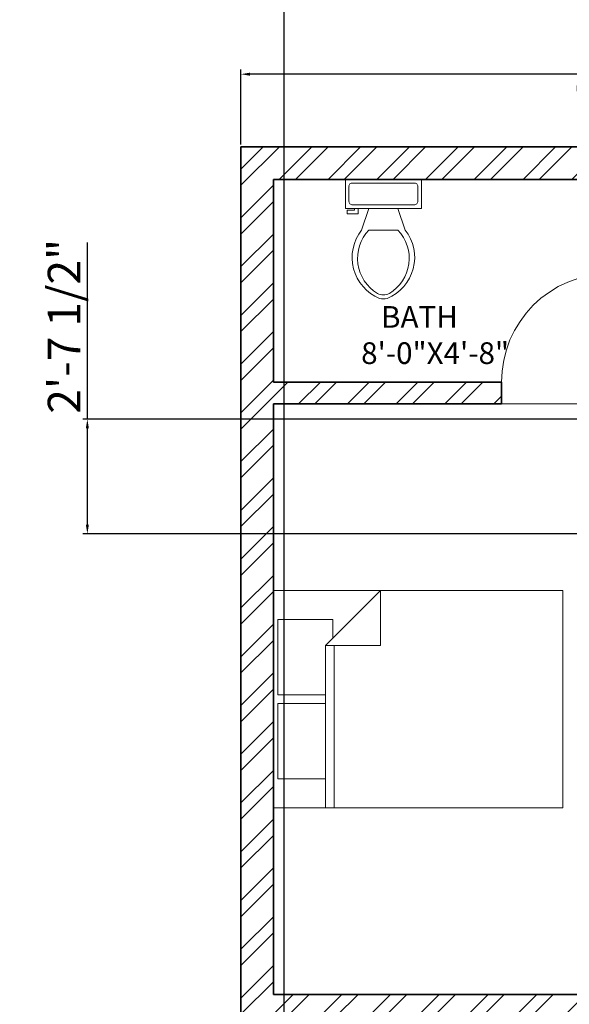
# Model space of a CAD drawing. Units: inches. Extents: x 744 to 1448, y 5126 to 6077.
# Tile 5 of 10: x 744 to 895, y 5585 to 5857. Entities that reach past the tile are written whole.
import ezdxf

# ---------------------------------------------------------------- set-up
doc = ezdxf.new("R2010")
doc.units = ezdxf.units.IN
for name, color, linetype, lineweight in [('A-ANNO-DIMS', 2, 'Continuous', 18), ('A-AREA-IDEN', 7, 'Continuous', 18), ('A-DOOR', 4, 'Continuous', 18), ('A-FLOR-FIXT', 9, 'Continuous', 18), ('A-FURN', 8, 'Continuous', 18), ('A-WALL', 7, 'Continuous', 35), ('A-WALL-PATT', 252, 'Continuous', 13)]:
    doc.layers.add(name, color=color, linetype=linetype, lineweight=lineweight)
doc.styles.get("Standard").update_dxf_attribs({"font": 'arial.ttf'})
doc.dimstyles.new('ISO-25', dxfattribs={"dimtxt": 9, "dimasz": 2.5, "dimexe": 1.25, "dimexo": 0.625, "dimtad": 1, "dimlunit": 3, "dimtxsty": 'Standard', "dimcen": 2.5, "dimadec": 0, "dimazin": 0, "dimtfac": 1, "dimtmove": 0, "dimatfit": 3, "dimfxl": 1, "dimarcsym": 0})

# ---------------------------------------------------------------- blocks, each defined once
blk = doc.blocks.new('*U4')
for p, q in [((0, 0), (0, 6)), ((40, 0), (40, 6))]:
    blk.add_line(p, q)
blk.add_lwpolyline([(0, 0), (0, -40), (1.75, -40), (1.75, 0)], close=True)
blk.add_arc((0, 0), 40, 270, 0)
blk = doc.blocks.new('*U8')
for p, q in [((9.5, -6), (9.5, -2)), ((-8, -8.5), (-8, -8)), ((-7, -8), (-7, -9.5)), ((-4, -8), (-6, -14)), ((4, -8), (6, -14)), ((-10, -8.5), (-8, -8.5)), ((-10, -9.5), (-10, -8.5)), ((-7, -9.5), (-10, -9.5)), ((4, -14), (-4, -14))]:
    blk.add_line(p, q)
blk.add_lwpolyline([(10.5, -8), (10.5, 0), (-10.5, 0), (-10.5, -8)], close=True)
for points in [[(-9.5, -2), (-9.5, -6)], [(8.5, -1), (-8.5, -1)], [(-8.5, -7), (8.5, -7)]]:
    blk.add_lwpolyline(points)
for centre, radius, start, end in [((-8.62, -1.88), 0.884, 81.8699, 188.1301), ((8.62, -1.88), 0.884, 351.8699, 98.1301), ((-8.62, -6.12), 0.884, 171.8699, 278.1301), ((8.62, -6.12), 0.884, 261.8699, 8.1301), ((3.52, -21.58), 12.17, 141.4691, 247.9714), ((4.2, -21.82), 11.33, 136.3677, 238.9468), ((-3.52, -21.58), 12.17, 292.0284, 38.5307), ((-4.2, -21.82), 11.33, 301.053, 43.6321), ((0, -27.88), 4, 245.7318, 294.2682), ((0, -29), 4, 254.8605, 285.1395)]:
    blk.add_arc(centre, radius, start, end)
blk = doc.blocks.new('Bed - Queen')
for p, q in [((0, -80.00003), (0, 0)), ((0, 0), (59.99999, 0)), ((59.99999, 0), (59.99999, -80.00003)), ((7.99999, -1.2), (28.79998, -1.2)), ((7.99999, -14.4), (7.99999, -1.2)), ((28.79998, -1.2), (28.79998, -14.4)), ((31.19999, -1.2), (51.99999, -1.2)), ((31.19999, -14.4), (31.19999, -1.2)), ((51.99999, -1.2), (51.99999, -16.4)), ((0, -14.4), (44.8, -14.4)), ((59.99999, -29.6), (44.8, -14.4)), ((44.8, -14.4), (44.8, -29.6)), ((44.8, -16.8), (0, -16.8)), ((51.99999, -16.4), (46.79936, -16.4)), ((44.8, -29.6), (59.99999, -29.6)), ((59.99999, -80.00003), (0, -80.00003))]:
    blk.add_line(p, q)
blk = doc.blocks.new('*D24')
at = {"layer": 'A-ANNO-DIMS', "color": 0, "lineweight": -2, "transparency": 16777216}
for p, q in [((804.68, 5822.44), (804.68, 5843.13)), ((1320.68, 5822.44), (1320.68, 5843.13)), ((1318.18, 5841.88), (807.18, 5841.88))]:
    blk.add_line(p, q, dxfattribs=at)
at = {"layer": 'A-ANNO-DIMS', "color": 0, "transparency": 16777216}
for points in [[(807.18, 5842.3), (807.18, 5841.46), (804.68, 5841.88)], [(1318.18, 5842.3), (1318.18, 5841.46), (1320.68, 5841.88)]]:
    blk.add_solid(points, dxfattribs=at)
at = {"layer": 'Defpoints', "color": 0, "transparency": 16777216}
for p in [(804.68, 5841.88), (804.68, 5821.82), (1320.68, 5821.82)]:
    blk.add_point(p, dxfattribs=at)
at = {"layer": 'A-ANNO-DIMS', "color": 0, "transparency": 16777216, "insert": (1062.68, 5847.1), "char_height": 9, "attachment_point": 5}
blk.add_mtext("43'", dxfattribs=at)
blk = doc.blocks.new('*D41')
at = {"layer": 'A-ANNO-DIMS', "color": 0, "lineweight": -2, "transparency": 16777216}
for p, q in [((908.53, 5795.32), (908.53, 5925.53)), ((911.06, 5795.32), (907.28, 5795.32)), ((908.53, 5776.82), (908.53, 5792.82)), ((911.06, 5774.32), (907.28, 5774.32))]:
    blk.add_line(p, q, dxfattribs=at)
at = {"layer": 'A-ANNO-DIMS', "color": 0, "transparency": 16777216}
for points in [[(908.12, 5792.82), (908.95, 5792.82), (908.53, 5795.32)], [(908.12, 5776.82), (908.95, 5776.82), (908.53, 5774.32)]]:
    blk.add_solid(points, dxfattribs=at)
at = {"layer": 'Defpoints', "color": 0, "transparency": 16777216}
for p in [(908.53, 5795.32), (911.68, 5795.32), (911.68, 5774.32)]:
    blk.add_point(p, dxfattribs=at)
at = {"layer": 'A-ANNO-DIMS', "color": 0, "transparency": 16777216, "insert": (903.25, 5861.67), "char_height": 9, "attachment_point": 5, "rotation": 90}
blk.add_mtext('WINDOW C 1\'-9" TYP.', dxfattribs=at)
blk = doc.blocks.new('*D59')
at = {"layer": 'A-ANNO-DIMS', "color": 0, "lineweight": -2, "transparency": 16777216}
for p, q in [((762.28, 5746.58), (762.28, 5795.38)), ((1128.24, 5746.58), (761.03, 5746.58)), ((762.28, 5717.4), (762.28, 5744.08)), ((1128.24, 5714.9), (761.03, 5714.9))]:
    blk.add_line(p, q, dxfattribs=at)
at = {"layer": 'A-ANNO-DIMS', "color": 0, "transparency": 16777216}
for points in [[(761.87, 5744.08), (762.7, 5744.08), (762.28, 5746.58)], [(761.87, 5717.4), (762.7, 5717.4), (762.28, 5714.9)]]:
    blk.add_solid(points, dxfattribs=at)
at = {"layer": 'Defpoints', "color": 0, "transparency": 16777216}
for p in [(762.28, 5746.58), (1128.86, 5746.58), (1128.86, 5714.9)]:
    blk.add_point(p, dxfattribs=at)
at = {"layer": 'A-ANNO-DIMS', "color": 0, "transparency": 16777216, "insert": (757.01, 5772.23), "char_height": 9, "attachment_point": 5, "rotation": 90}
blk.add_mtext('2\'-7 1/2"', dxfattribs=at)
blk = doc.blocks.new('*D62')
at = {"layer": 'A-ANNO-DIMS', "color": 0, "lineweight": -2, "transparency": 16777216}
for p, q in [((816.68, 5262.94), (816.68, 6059.61)), ((819.18, 6058.36), (974.68, 6058.36)), ((977.18, 5262.94), (977.18, 6059.61))]:
    blk.add_line(p, q, dxfattribs=at)
at = {"layer": 'A-ANNO-DIMS', "color": 0, "transparency": 16777216}
for points in [[(819.18, 6058.78), (819.18, 6057.95), (816.68, 6058.36)], [(974.68, 6058.78), (974.68, 6057.95), (977.18, 6058.36)]]:
    blk.add_solid(points, dxfattribs=at)
at = {"layer": 'Defpoints', "color": 0, "transparency": 16777216}
for p in [(977.18, 6058.36), (816.68, 5262.32), (977.18, 5262.32)]:
    blk.add_point(p, dxfattribs=at)
at = {"layer": 'A-ANNO-DIMS', "color": 0, "transparency": 16777216, "insert": (896.93, 6063.64), "char_height": 9, "attachment_point": 5}
blk.add_mtext('13\'-4 1/2"', dxfattribs=at)

msp = doc.modelspace()

# ---------------------------------------------------------------- hatches: boundary and pattern name
at = {"layer": 'A-WALL-PATT'}
h = msp.add_hatch(dxfattribs=at)
h.set_pattern_fill('ANSI32', color=256)
h.paths.add_polyline_path([(813.684, 5750.816), (876.684, 5750.816), (876.684, 5756.816), (813.684, 5756.816), (813.684, 5812.816), (909.684, 5812.816), (909.684, 5795.316), (915.684, 5795.316), (915.684, 5812.816), (1209.684, 5812.816), (1209.684, 5795.316), (1215.684, 5795.316), (1215.684, 5812.816), (1311.684, 5812.816), (1311.684, 5756.816), (1248.684, 5756.816), (1248.684, 5750.816), (1311.684, 5750.816), (1311.684, 5570.816), (1179.044, 5570.816), (1179.044, 5564.816), (1311.684, 5564.816), (1311.684, 5383.316), (1260.684, 5383.316), (1260.684, 5377.316), (1311.684, 5377.316), (1311.684, 5320.316), (1227.684, 5320.316), (1227.684, 5333.816), (1221.684, 5333.816), (1221.684, 5314.316), (1320.684, 5314.316), (1320.684, 5821.816), (804.684, 5821.816), (804.684, 5472.316), (926.184, 5472.316), (926.184, 5481.316), (813.684, 5481.316), (813.684, 5581.616), (946.284, 5581.616), (946.284, 5587.616), (813.684, 5587.616)])
h.paths.add_polyline_path([(1155.684, 5525.816), (1149.684, 5525.816), (1149.684, 5481.316), (1025.184, 5481.316), (1025.184, 5475.316), (1146.684, 5475.316), (1146.684, 5323.316), (1118.788, 5323.316), (1118.788, 5314.316), (1146.684, 5314.316), (1155.684, 5314.316), (1155.684, 5374.316), (1170.35, 5374.316), (1170.35, 5383.316), (1155.684, 5383.316)], flags=17)
h.paths.add_polyline_path([(1230.684, 5383.316), (1213.35, 5383.316), (1213.35, 5374.316), (1221.684, 5374.316), (1221.684, 5363.816), (1226.184, 5363.816), (1227.684, 5363.816), (1227.684, 5377.316), (1230.684, 5377.316)], flags=17)
h.paths.add_polyline_path([(1185.684, 5671.816), (1155.684, 5671.816), (1155.684, 5750.816), (1161.575, 5750.816), (1161.575, 5756.816), (1157.542, 5756.816), (1157.847, 5756.715), (1155.79, 5756.816), (1149.684, 5756.816), (1149.684, 5750.816), (1149.684, 5671.816), (1121.684, 5671.816), (1121.684, 5665.816), (1179.684, 5665.816), (1179.684, 5609.816), (1185.684, 5609.816)], flags=17)
h.paths.add_polyline_path([(1003.684, 5671.816), (975.684, 5671.816), (975.684, 5750.816), (975.684, 5756.816), (965.205, 5756.816), (965.205, 5750.816), (969.684, 5750.816), (969.684, 5671.816), (939.684, 5671.816), (939.684, 5626.616), (945.684, 5626.616), (945.684, 5665.816), (1003.684, 5665.816)], flags=17)
h.paths.add_polyline_path([(915.684, 5774.316), (909.684, 5774.316), (909.684, 5756.816), (906.684, 5756.816), (906.684, 5752.316), (906.684, 5750.816), (922.205, 5750.816), (922.205, 5756.816), (915.684, 5756.816)], flags=17)
h.paths.add_polyline_path([(1215.684, 5774.316), (1209.684, 5774.316), (1209.684, 5756.816), (1204.575, 5756.816), (1204.575, 5750.816), (1218.684, 5750.816), (1218.684, 5756.816), (1215.684, 5756.816)], flags=17)
h.paths.add_polyline_path([(1063.788, 5323.316), (1025.184, 5323.316), (1025.184, 5314.316), (1063.788, 5314.316)])
h.paths.add_polyline_path([(986.184, 5475.316), (989.184, 5475.316), (989.184, 5481.316), (974.184, 5481.316), (974.184, 5475.916), (974.184, 5472.316), (977.184, 5472.316), (977.184, 5314.316), (989.184, 5314.316), (989.184, 5319.716), (989.184, 5323.316), (986.184, 5323.316)])

# ---------------------------------------------------------------- linework, layer by layer
at = {"layer": 'A-DOOR'}
msp.add_line((876.684, 5750.816), (906.684, 5750.816), dxfattribs=at)
at = {"layer": 'A-WALL'}
for p, q in [((804.684, 5250.316), (804.684, 5821.816)), ((804.684, 5821.816), (1320.684, 5821.816)), ((813.684, 5812.816), (909.684, 5812.816)), ((813.684, 5756.816), (813.684, 5812.816)), ((813.684, 5756.816), (876.684, 5756.816)), ((876.684, 5756.816), (876.684, 5750.816)), ((813.684, 5750.816), (876.684, 5750.816)), ((813.684, 5587.616), (813.684, 5750.816)), ((813.684, 5587.616), (946.284, 5587.616))]:
    msp.add_line(p, q, dxfattribs=at)

# ---------------------------------------------------------------- block references
at = {"layer": 'A-DOOR', "xscale": 0.75, "yscale": 0.75, "zscale": 0.75, "rotation": 180.0000000000004}
msp.add_blockref('*U4', (906.684, 5756.816), dxfattribs=at)
at = {"layer": 'A-FLOR-FIXT'}
msp.add_blockref('*U8', (844.062, 5812.816), dxfattribs=at)
at = {"layer": 'A-FURN', "rotation": 89.99999999999999}
msp.add_blockref('Bed - Queen', (813.684, 5639.216), dxfattribs=at)

# ---------------------------------------------------------------- texts
at = {"layer": 'A-AREA-IDEN', "insert": (837.92, 5777.819), "char_height": 6, "attachment_point": 1}
msp.add_mtext_dynamic_manual_height_columns('   BATH\\P8\'-0"X4\'-8"', width=39.96322, gutter_width=12.5, heights=[0], dxfattribs=at)

# ---------------------------------------------------------------- dimensions: what is measured, and where the dimension line sits
at = {"layer": 'A-ANNO-DIMS'}
for base, p1, p2, override, picture, middle in [((977.184, 6058.363), (816.684, 5262.316), (977.184, 5262.316), {"dimdec": 1, "dimlfac": 1, "dimrnd": 0, "dimzin": 1, "dimdsep": 46, "dimlunit": 4, "dimfrac": 2}, '*D62', (896.934, 6063.645)), ((804.684, 5841.882), (1320.684, 5821.816), (804.684, 5821.816), {"dimclrd": 0, "dimclre": 0, "dimclrt": 0}, '*D24', (1062.684, 5847.105))]:
    dim = msp.add_linear_dim(base=base, p1=p1, p2=p2, dimstyle='ISO-25', override=override, dxfattribs=at)
    dim.commit()
    dim.dimension.update_dxf_attribs({"geometry": picture, "text_midpoint": middle})
dim = msp.add_linear_dim(base=(908.534, 5795.316), p1=(911.684, 5774.316), p2=(911.684, 5795.316), angle=90, text='WINDOW C <> TYP.', dimstyle='ISO-25', override={"dimdec": 1, "dimlfac": 1, "dimrnd": 0, "dimzin": 1, "dimdsep": 46, "dimlunit": 4, "dimfrac": 2}, dxfattribs=at)
dim.commit()
dim.dimension.update_dxf_attribs({"geometry": '*D41', "text_midpoint": (903.253, 5861.671)})
dim = msp.add_linear_dim(base=(762.284, 5746.584), p1=(1128.864, 5714.896), p2=(1128.864, 5746.584), angle=90, dimstyle='ISO-25', override={"dimdec": 1, "dimlfac": 1, "dimrnd": 0, "dimzin": 1, "dimdsep": 46, "dimlunit": 4, "dimfrac": 2}, dxfattribs=at)
dim.commit()
dim.dimension.update_dxf_attribs({"geometry": '*D59', "text_midpoint": (757.006, 5772.234)})

doc.saveas('drawing.dxf')
